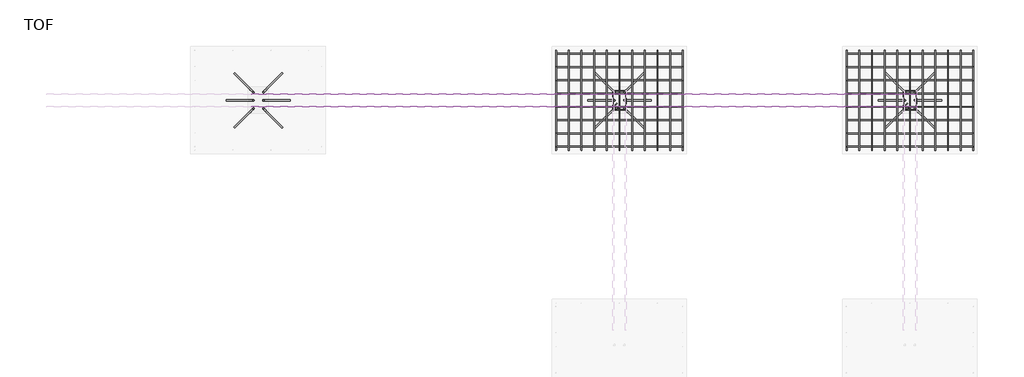
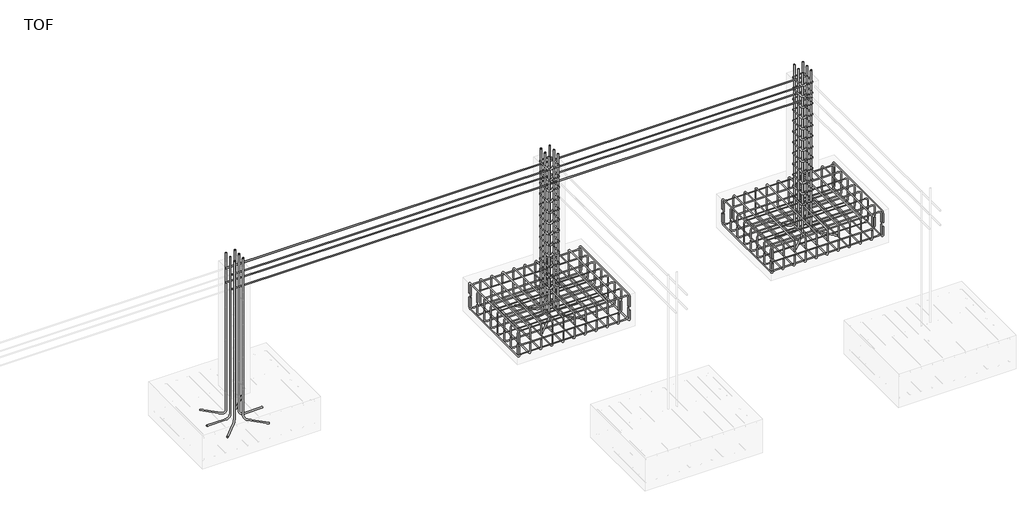
# One storey, part 10 of 10: 36 reinforcing bars.
"""IFC4 building model written with IfcOpenShell, lengths in millimetres."""

from ifc_helpers import new_model, si_unit, point, frame, origin, place, context, project, spatial, polyline, circle_curve, trimmed, segment, composite_curve, source, transform, mapped, element, save
from ifc_brep_helpers import swept_disk

model = new_model("IFC4")

# Units and contexts
model_context = context("Model", 3, world=origin())
ifc_project = project(units=[si_unit("LENGTHUNIT", "METRE", prefix="MILLI")], contexts=[model_context])

# Site, building, storey
site = spatial("IfcSite", under=ifc_project)
building = spatial("IfcBuilding", under=site)
storey = spatial("IfcBuildingStorey", under=building, Name="TOF", Elevation=-1828.8)

# Reinforcing bars
placement = place(None, origin())
reinforcing_bar_shape = source(origin(), model_context, "Body", "SolidModel", [
    swept_disk(composite_curve([segment(polyline([(10345.2782143, -7144.6267376, -2018.8), (10345.2782143, -7144.6267376, -1908.8)]), True, "CONTINUOUS"), segment(trimmed(circle_curve(frame((10345.2782143, -7179.6267376, -1908.8), z_axis=(1.0, 0.0, 0.0), x_axis=(0.0, 35.0, 0.0)), 35.0), [point((10345.2782143, -7144.6267376, -1908.8))], [point((10345.2782143, -7179.6267376, -1873.8))], True, "CARTESIAN"), True, "CONTINUOUS"), segment(polyline([(10345.2782143, -7179.6267376, -1873.8), (10345.2782143, -8219.6267376, -1873.8)]), True, "CONTINUOUS"), segment(trimmed(circle_curve(frame((10345.2782143, -8219.6267376, -1908.8), z_axis=(1.0, 0.0, 0.0), x_axis=(0.0, 0.0, 35.0)), 35.0), [point((10345.2782143, -8219.6267376, -1873.8))], [point((10345.2782143, -8254.6267376, -1908.8))], True, "CARTESIAN"), True, "CONTINUOUS"), segment(polyline([(10345.2782143, -8254.6267376, -1908.8), (10345.2782143, -8254.6267376, -2018.8)]), True, "CONTINUOUS")], self_intersect=False), 5.0),
])
element("IfcReinforcingBar", 1, at=placement, inside=storey, context=model_context, shape_type="MappedRepresentation", body=[
    mapped(reinforcing_bar_shape, transform((0.0, 0.0, 0.0), x_axis=(1.0, 0.0, 0.0), y_axis=(0.0, 1.0, 0.0), z_axis=(0.0, 0.0, 1.0))),
    mapped(reinforcing_bar_shape, transform((-141.0, 0.0, 0.0), x_axis=(1.0, 0.0, 0.0), y_axis=(0.0, 1.0, 0.0), z_axis=(0.0, 0.0, 1.0))),
    mapped(reinforcing_bar_shape, transform((-282.0, 0.0, 0.0), x_axis=(1.0, 0.0, 0.0), y_axis=(0.0, 1.0, 0.0), z_axis=(0.0, 0.0, 1.0))),
    mapped(reinforcing_bar_shape, transform((-423.0, 0.0, 0.0), x_axis=(1.0, 0.0, 0.0), y_axis=(0.0, 1.0, 0.0), z_axis=(0.0, 0.0, 1.0))),
    mapped(reinforcing_bar_shape, transform((-564.0, 0.0, 0.0), x_axis=(1.0, 0.0, 0.0), y_axis=(0.0, 1.0, 0.0), z_axis=(0.0, 0.0, 1.0))),
    mapped(reinforcing_bar_shape, transform((-705.0, 0.0, 0.0), x_axis=(1.0, 0.0, 0.0), y_axis=(0.0, 1.0, 0.0), z_axis=(0.0, 0.0, 1.0))),
    mapped(reinforcing_bar_shape, transform((-846.0, 0.0, 0.0), x_axis=(1.0, 0.0, 0.0), y_axis=(0.0, 1.0, 0.0), z_axis=(0.0, 0.0, 1.0))),
    mapped(reinforcing_bar_shape, transform((-987.0, 0.0, 0.0), x_axis=(1.0, 0.0, 0.0), y_axis=(0.0, 1.0, 0.0), z_axis=(0.0, 0.0, 1.0))),
    mapped(reinforcing_bar_shape, transform((-1128.0, 0.0, 0.0), x_axis=(1.0, 0.0, 0.0), y_axis=(0.0, 1.0, 0.0), z_axis=(0.0, 0.0, 1.0))),
    mapped(reinforcing_bar_shape, transform((-1269.0, 0.0, 0.0), x_axis=(1.0, 0.0, 0.0), y_axis=(0.0, 1.0, 0.0), z_axis=(0.0, 0.0, 1.0))),
    mapped(reinforcing_bar_shape, transform((-1410.0, 0.0, 0.0), x_axis=(1.0, 0.0, 0.0), y_axis=(0.0, 1.0, 0.0), z_axis=(0.0, 0.0, 1.0))),
])
reinforcing_bar_2_shape = source(origin(), model_context, "Body", "SolidModel", [
    swept_disk(composite_curve([segment(polyline([(10345.2782143, -8254.6267376, -2077.5233378), (10345.2782143, -8254.6267376, -2187.5233378)]), True, "CONTINUOUS"), segment(trimmed(circle_curve(frame((10345.2782143, -8219.6267376, -2187.5233378), z_axis=(1.0, 0.0, 0.0), x_axis=(0.0, -35.0, 0.0)), 35.0), [point((10345.2782143, -8254.6267376, -2187.5233378))], [point((10345.2782143, -8219.6267376, -2222.5233378))], True, "CARTESIAN"), True, "CONTINUOUS"), segment(polyline([(10345.2782143, -8219.6267376, -2222.5233378), (10345.2782143, -7179.6267376, -2222.5233378)]), True, "CONTINUOUS"), segment(trimmed(circle_curve(frame((10345.2782143, -7179.6267376, -2187.5233378), z_axis=(1.0, 0.0, 0.0), x_axis=(0.0, 0.0, -35.0)), 35.0), [point((10345.2782143, -7179.6267376, -2222.5233378))], [point((10345.2782143, -7144.6267376, -2187.5233378))], True, "CARTESIAN"), True, "CONTINUOUS"), segment(polyline([(10345.2782143, -7144.6267376, -2187.5233378), (10345.2782143, -7144.6267376, -2077.5233378)]), True, "CONTINUOUS")], self_intersect=False), 5.0),
])
element("IfcReinforcingBar", 2, at=placement, inside=storey, context=model_context, shape_type="MappedRepresentation", body=[
    mapped(reinforcing_bar_2_shape, transform((0.0, 0.0, 0.0), x_axis=(1.0, 0.0, 0.0), y_axis=(0.0, 1.0, 0.0), z_axis=(0.0, 0.0, 1.0))),
    mapped(reinforcing_bar_2_shape, transform((-141.0, 0.0, 0.0), x_axis=(1.0, 0.0, 0.0), y_axis=(0.0, 1.0, 0.0), z_axis=(0.0, 0.0, 1.0))),
    mapped(reinforcing_bar_2_shape, transform((-282.0, 0.0, 0.0), x_axis=(1.0, 0.0, 0.0), y_axis=(0.0, 1.0, 0.0), z_axis=(0.0, 0.0, 1.0))),
    mapped(reinforcing_bar_2_shape, transform((-423.0, 0.0, 0.0), x_axis=(1.0, 0.0, 0.0), y_axis=(0.0, 1.0, 0.0), z_axis=(0.0, 0.0, 1.0))),
    mapped(reinforcing_bar_2_shape, transform((-564.0, 0.0, 0.0), x_axis=(1.0, 0.0, 0.0), y_axis=(0.0, 1.0, 0.0), z_axis=(0.0, 0.0, 1.0))),
    mapped(reinforcing_bar_2_shape, transform((-705.0, 0.0, 0.0), x_axis=(1.0, 0.0, 0.0), y_axis=(0.0, 1.0, 0.0), z_axis=(0.0, 0.0, 1.0))),
    mapped(reinforcing_bar_2_shape, transform((-846.0, 0.0, 0.0), x_axis=(1.0, 0.0, 0.0), y_axis=(0.0, 1.0, 0.0), z_axis=(0.0, 0.0, 1.0))),
    mapped(reinforcing_bar_2_shape, transform((-987.0, 0.0, 0.0), x_axis=(1.0, 0.0, 0.0), y_axis=(0.0, 1.0, 0.0), z_axis=(0.0, 0.0, 1.0))),
    mapped(reinforcing_bar_2_shape, transform((-1128.0, 0.0, 0.0), x_axis=(1.0, 0.0, 0.0), y_axis=(0.0, 1.0, 0.0), z_axis=(0.0, 0.0, 1.0))),
    mapped(reinforcing_bar_2_shape, transform((-1269.0, 0.0, 0.0), x_axis=(1.0, 0.0, 0.0), y_axis=(0.0, 1.0, 0.0), z_axis=(0.0, 0.0, 1.0))),
    mapped(reinforcing_bar_2_shape, transform((-1410.0, 0.0, 0.0), x_axis=(1.0, 0.0, 0.0), y_axis=(0.0, 1.0, 0.0), z_axis=(0.0, 0.0, 1.0))),
])
reinforcing_bar_3_shape = source(origin(), model_context, "Body", "SolidModel", [
    swept_disk(composite_curve([segment(polyline([(10345.2782143, -7179.6861459, -2066.1776706), (10345.2782143, -7179.6861459, -2176.1776706)]), True, "CONTINUOUS"), segment(trimmed(circle_curve(frame((10310.2782143, -7179.6861459, -2176.1776706), z_axis=(0.0, 1.0, 0.0), x_axis=(35.0, 0.0, 0.0)), 35.0), [point((10345.2782143, -7179.6861459, -2176.1776706))], [point((10310.2782143, -7179.6861459, -2211.1776706))], True, "CARTESIAN"), True, "CONTINUOUS"), segment(polyline([(10310.2782143, -7179.6861459, -2211.1776706), (8970.2782143, -7179.6861459, -2211.1776706)]), True, "CONTINUOUS"), segment(trimmed(circle_curve(frame((8970.2782143, -7179.6861459, -2176.1776706), z_axis=(0.0, 1.0, 0.0), x_axis=(0.0, 0.0, -35.0)), 35.0), [point((8970.2782143, -7179.6861459, -2211.1776706))], [point((8935.2782143, -7179.6861459, -2176.1776706))], True, "CARTESIAN"), True, "CONTINUOUS"), segment(polyline([(8935.2782143, -7179.6861459, -2176.1776706), (8935.2782143, -7179.6861459, -2066.1776706)]), True, "CONTINUOUS")], self_intersect=False), 5.0),
])
element("IfcReinforcingBar", 3, at=placement, inside=storey, context=model_context, shape_type="MappedRepresentation", body=[
    mapped(reinforcing_bar_3_shape, transform((0.0, 0.0, 0.0), x_axis=(1.0, 0.0, 0.0), y_axis=(0.0, 1.0, 0.0), z_axis=(0.0, 0.0, 1.0))),
    mapped(reinforcing_bar_3_shape, transform((0.0, -148.0321606, 0.0), x_axis=(1.0, 0.0, 0.0), y_axis=(0.0, 1.0, 0.0), z_axis=(0.0, 0.0, 1.0))),
    mapped(reinforcing_bar_3_shape, transform((0.0, -296.0643211, 0.0), x_axis=(1.0, 0.0, 0.0), y_axis=(0.0, 1.0, 0.0), z_axis=(0.0, 0.0, 1.0))),
    mapped(reinforcing_bar_3_shape, transform((0.0, -444.0964817, 0.0), x_axis=(1.0, 0.0, 0.0), y_axis=(0.0, 1.0, 0.0), z_axis=(0.0, 0.0, 1.0))),
    mapped(reinforcing_bar_3_shape, transform((0.0, -592.1286423, 0.0), x_axis=(1.0, 0.0, 0.0), y_axis=(0.0, 1.0, 0.0), z_axis=(0.0, 0.0, 1.0))),
    mapped(reinforcing_bar_3_shape, transform((0.0, -740.1608029, 0.0), x_axis=(1.0, 0.0, 0.0), y_axis=(0.0, 1.0, 0.0), z_axis=(0.0, 0.0, 1.0))),
    mapped(reinforcing_bar_3_shape, transform((0.0, -888.1929634, 0.0), x_axis=(1.0, 0.0, 0.0), y_axis=(0.0, 1.0, 0.0), z_axis=(0.0, 0.0, 1.0))),
    mapped(reinforcing_bar_3_shape, transform((0.0, -1036.225124, 0.0), x_axis=(1.0, 0.0, 0.0), y_axis=(0.0, 1.0, 0.0), z_axis=(0.0, 0.0, 1.0))),
])
reinforcing_bar_4_shape = source(origin(), model_context, "Body", "SolidModel", [
    swept_disk(composite_curve([segment(polyline([(10345.2782143, -8215.9112699, -2039.256778), (10345.2782143, -8215.9112699, -1929.256778)]), True, "CONTINUOUS"), segment(trimmed(circle_curve(frame((10310.2782143, -8215.9112699, -1929.256778), z_axis=(0.0, -1.0, 0.0), x_axis=(35.0, 0.0, 0.0)), 35.0), [point((10345.2782143, -8215.9112699, -1929.256778))], [point((10310.2782143, -8215.9112699, -1894.256778))], True, "CARTESIAN"), True, "CONTINUOUS"), segment(polyline([(10310.2782143, -8215.9112699, -1894.256778), (8970.2782143, -8215.9112699, -1894.256778)]), True, "CONTINUOUS"), segment(trimmed(circle_curve(frame((8970.2782143, -8215.9112699, -1929.256778), z_axis=(0.0, -1.0, 0.0), x_axis=(0.0, 0.0, 35.0)), 35.0), [point((8970.2782143, -8215.9112699, -1894.256778))], [point((8935.2782143, -8215.9112699, -1929.256778))], True, "CARTESIAN"), True, "CONTINUOUS"), segment(polyline([(8935.2782143, -8215.9112699, -1929.256778), (8935.2782143, -8215.9112699, -2039.256778)]), True, "CONTINUOUS")], self_intersect=False), 5.0),
])
element("IfcReinforcingBar", 4, at=placement, inside=storey, context=model_context, shape_type="MappedRepresentation", body=[
    mapped(reinforcing_bar_4_shape, transform((0.0, 0.0, 0.0), x_axis=(1.0, 0.0, 0.0), y_axis=(0.0, 1.0, 0.0), z_axis=(0.0, 0.0, 1.0))),
    mapped(reinforcing_bar_4_shape, transform((0.0, 148.0321606, 0.0), x_axis=(1.0, 0.0, 0.0), y_axis=(0.0, 1.0, 0.0), z_axis=(0.0, 0.0, 1.0))),
    mapped(reinforcing_bar_4_shape, transform((0.0, 296.0643211, 0.0), x_axis=(1.0, 0.0, 0.0), y_axis=(0.0, 1.0, 0.0), z_axis=(0.0, 0.0, 1.0))),
    mapped(reinforcing_bar_4_shape, transform((0.0, 444.0964817, 0.0), x_axis=(1.0, 0.0, 0.0), y_axis=(0.0, 1.0, 0.0), z_axis=(0.0, 0.0, 1.0))),
    mapped(reinforcing_bar_4_shape, transform((0.0, 592.1286423, 0.0), x_axis=(1.0, 0.0, 0.0), y_axis=(0.0, 1.0, 0.0), z_axis=(0.0, 0.0, 1.0))),
    mapped(reinforcing_bar_4_shape, transform((0.0, 740.1608029, 0.0), x_axis=(1.0, 0.0, 0.0), y_axis=(0.0, 1.0, 0.0), z_axis=(0.0, 0.0, 1.0))),
    mapped(reinforcing_bar_4_shape, transform((0.0, 888.1929634, 0.0), x_axis=(1.0, 0.0, 0.0), y_axis=(0.0, 1.0, 0.0), z_axis=(0.0, 0.0, 1.0))),
    mapped(reinforcing_bar_4_shape, transform((0.0, 1036.225124, 0.0), x_axis=(1.0, 0.0, 0.0), y_axis=(0.0, 1.0, 0.0), z_axis=(0.0, 0.0, 1.0))),
])
reinforcing_bar_5_shape = source(origin(), model_context, "Body", "SolidModel", [
    swept_disk(composite_curve([segment(polyline([(13575.2782143, -7144.6267376, -2018.8), (13575.2782143, -7144.6267376, -1908.8)]), True, "CONTINUOUS"), segment(trimmed(circle_curve(frame((13575.2782143, -7179.6267376, -1908.8), z_axis=(1.0, 0.0, 0.0), x_axis=(0.0, 35.0, 0.0)), 35.0), [point((13575.2782143, -7144.6267376, -1908.8))], [point((13575.2782143, -7179.6267376, -1873.8))], True, "CARTESIAN"), True, "CONTINUOUS"), segment(polyline([(13575.2782143, -7179.6267376, -1873.8), (13575.2782143, -8219.6267376, -1873.8)]), True, "CONTINUOUS"), segment(trimmed(circle_curve(frame((13575.2782143, -8219.6267376, -1908.8), z_axis=(1.0, 0.0, 0.0), x_axis=(0.0, 0.0, 35.0)), 35.0), [point((13575.2782143, -8219.6267376, -1873.8))], [point((13575.2782143, -8254.6267376, -1908.8))], True, "CARTESIAN"), True, "CONTINUOUS"), segment(polyline([(13575.2782143, -8254.6267376, -1908.8), (13575.2782143, -8254.6267376, -2018.8)]), True, "CONTINUOUS")], self_intersect=False), 5.0),
])
element("IfcReinforcingBar", 5, at=placement, inside=storey, context=model_context, shape_type="MappedRepresentation", body=[
    mapped(reinforcing_bar_5_shape, transform((0.0, 0.0, 0.0), x_axis=(1.0, 0.0, 0.0), y_axis=(0.0, 1.0, 0.0), z_axis=(0.0, 0.0, 1.0))),
    mapped(reinforcing_bar_5_shape, transform((-141.0, 0.0, 0.0), x_axis=(1.0, 0.0, 0.0), y_axis=(0.0, 1.0, 0.0), z_axis=(0.0, 0.0, 1.0))),
    mapped(reinforcing_bar_5_shape, transform((-282.0, 0.0, 0.0), x_axis=(1.0, 0.0, 0.0), y_axis=(0.0, 1.0, 0.0), z_axis=(0.0, 0.0, 1.0))),
    mapped(reinforcing_bar_5_shape, transform((-423.0, 0.0, 0.0), x_axis=(1.0, 0.0, 0.0), y_axis=(0.0, 1.0, 0.0), z_axis=(0.0, 0.0, 1.0))),
    mapped(reinforcing_bar_5_shape, transform((-564.0, 0.0, 0.0), x_axis=(1.0, 0.0, 0.0), y_axis=(0.0, 1.0, 0.0), z_axis=(0.0, 0.0, 1.0))),
    mapped(reinforcing_bar_5_shape, transform((-705.0, 0.0, 0.0), x_axis=(1.0, 0.0, 0.0), y_axis=(0.0, 1.0, 0.0), z_axis=(0.0, 0.0, 1.0))),
    mapped(reinforcing_bar_5_shape, transform((-846.0, 0.0, 0.0), x_axis=(1.0, 0.0, 0.0), y_axis=(0.0, 1.0, 0.0), z_axis=(0.0, 0.0, 1.0))),
    mapped(reinforcing_bar_5_shape, transform((-987.0, 0.0, 0.0), x_axis=(1.0, 0.0, 0.0), y_axis=(0.0, 1.0, 0.0), z_axis=(0.0, 0.0, 1.0))),
    mapped(reinforcing_bar_5_shape, transform((-1128.0, 0.0, 0.0), x_axis=(1.0, 0.0, 0.0), y_axis=(0.0, 1.0, 0.0), z_axis=(0.0, 0.0, 1.0))),
    mapped(reinforcing_bar_5_shape, transform((-1269.0, 0.0, 0.0), x_axis=(1.0, 0.0, 0.0), y_axis=(0.0, 1.0, 0.0), z_axis=(0.0, 0.0, 1.0))),
    mapped(reinforcing_bar_5_shape, transform((-1410.0, 0.0, 0.0), x_axis=(1.0, 0.0, 0.0), y_axis=(0.0, 1.0, 0.0), z_axis=(0.0, 0.0, 1.0))),
])
reinforcing_bar_6_shape = source(origin(), model_context, "Body", "SolidModel", [
    swept_disk(composite_curve([segment(polyline([(13575.2782143, -8254.6267376, -2077.5233378), (13575.2782143, -8254.6267376, -2187.5233378)]), True, "CONTINUOUS"), segment(trimmed(circle_curve(frame((13575.2782143, -8219.6267376, -2187.5233378), z_axis=(1.0, 0.0, 0.0), x_axis=(0.0, -35.0, 0.0)), 35.0), [point((13575.2782143, -8254.6267376, -2187.5233378))], [point((13575.2782143, -8219.6267376, -2222.5233378))], True, "CARTESIAN"), True, "CONTINUOUS"), segment(polyline([(13575.2782143, -8219.6267376, -2222.5233378), (13575.2782143, -7179.6267376, -2222.5233378)]), True, "CONTINUOUS"), segment(trimmed(circle_curve(frame((13575.2782143, -7179.6267376, -2187.5233378), z_axis=(1.0, 0.0, 0.0), x_axis=(0.0, 0.0, -35.0)), 35.0), [point((13575.2782143, -7179.6267376, -2222.5233378))], [point((13575.2782143, -7144.6267376, -2187.5233378))], True, "CARTESIAN"), True, "CONTINUOUS"), segment(polyline([(13575.2782143, -7144.6267376, -2187.5233378), (13575.2782143, -7144.6267376, -2077.5233378)]), True, "CONTINUOUS")], self_intersect=False), 5.0),
])
element("IfcReinforcingBar", 6, at=placement, inside=storey, context=model_context, shape_type="MappedRepresentation", body=[
    mapped(reinforcing_bar_6_shape, transform((0.0, 0.0, 0.0), x_axis=(1.0, 0.0, 0.0), y_axis=(0.0, 1.0, 0.0), z_axis=(0.0, 0.0, 1.0))),
    mapped(reinforcing_bar_6_shape, transform((-141.0, 0.0, 0.0), x_axis=(1.0, 0.0, 0.0), y_axis=(0.0, 1.0, 0.0), z_axis=(0.0, 0.0, 1.0))),
    mapped(reinforcing_bar_6_shape, transform((-282.0, 0.0, 0.0), x_axis=(1.0, 0.0, 0.0), y_axis=(0.0, 1.0, 0.0), z_axis=(0.0, 0.0, 1.0))),
    mapped(reinforcing_bar_6_shape, transform((-423.0, 0.0, 0.0), x_axis=(1.0, 0.0, 0.0), y_axis=(0.0, 1.0, 0.0), z_axis=(0.0, 0.0, 1.0))),
    mapped(reinforcing_bar_6_shape, transform((-564.0, 0.0, 0.0), x_axis=(1.0, 0.0, 0.0), y_axis=(0.0, 1.0, 0.0), z_axis=(0.0, 0.0, 1.0))),
    mapped(reinforcing_bar_6_shape, transform((-705.0, 0.0, 0.0), x_axis=(1.0, 0.0, 0.0), y_axis=(0.0, 1.0, 0.0), z_axis=(0.0, 0.0, 1.0))),
    mapped(reinforcing_bar_6_shape, transform((-846.0, 0.0, 0.0), x_axis=(1.0, 0.0, 0.0), y_axis=(0.0, 1.0, 0.0), z_axis=(0.0, 0.0, 1.0))),
    mapped(reinforcing_bar_6_shape, transform((-987.0, 0.0, 0.0), x_axis=(1.0, 0.0, 0.0), y_axis=(0.0, 1.0, 0.0), z_axis=(0.0, 0.0, 1.0))),
    mapped(reinforcing_bar_6_shape, transform((-1128.0, 0.0, 0.0), x_axis=(1.0, 0.0, 0.0), y_axis=(0.0, 1.0, 0.0), z_axis=(0.0, 0.0, 1.0))),
    mapped(reinforcing_bar_6_shape, transform((-1269.0, 0.0, 0.0), x_axis=(1.0, 0.0, 0.0), y_axis=(0.0, 1.0, 0.0), z_axis=(0.0, 0.0, 1.0))),
    mapped(reinforcing_bar_6_shape, transform((-1410.0, 0.0, 0.0), x_axis=(1.0, 0.0, 0.0), y_axis=(0.0, 1.0, 0.0), z_axis=(0.0, 0.0, 1.0))),
])
reinforcing_bar_7_shape = source(origin(), model_context, "Body", "SolidModel", [
    swept_disk(composite_curve([segment(polyline([(13575.2782143, -7179.6861459, -2066.1776706), (13575.2782143, -7179.6861459, -2176.1776706)]), True, "CONTINUOUS"), segment(trimmed(circle_curve(frame((13540.2782143, -7179.6861459, -2176.1776706), z_axis=(0.0, 1.0, 0.0), x_axis=(35.0, 0.0, 0.0)), 35.0), [point((13575.2782143, -7179.6861459, -2176.1776706))], [point((13540.2782143, -7179.6861459, -2211.1776706))], True, "CARTESIAN"), True, "CONTINUOUS"), segment(polyline([(13540.2782143, -7179.6861459, -2211.1776706), (12200.2782143, -7179.6861459, -2211.1776706)]), True, "CONTINUOUS"), segment(trimmed(circle_curve(frame((12200.2782143, -7179.6861459, -2176.1776706), z_axis=(0.0, 1.0, 0.0), x_axis=(0.0, 0.0, -35.0)), 35.0), [point((12200.2782143, -7179.6861459, -2211.1776706))], [point((12165.2782143, -7179.6861459, -2176.1776706))], True, "CARTESIAN"), True, "CONTINUOUS"), segment(polyline([(12165.2782143, -7179.6861459, -2176.1776706), (12165.2782143, -7179.6861459, -2066.1776706)]), True, "CONTINUOUS")], self_intersect=False), 5.0),
])
element("IfcReinforcingBar", 7, at=placement, inside=storey, context=model_context, shape_type="MappedRepresentation", body=[
    mapped(reinforcing_bar_7_shape, transform((0.0, 0.0, 0.0), x_axis=(1.0, 0.0, 0.0), y_axis=(0.0, 1.0, 0.0), z_axis=(0.0, 0.0, 1.0))),
    mapped(reinforcing_bar_7_shape, transform((0.0, -148.0321606, 0.0), x_axis=(1.0, 0.0, 0.0), y_axis=(0.0, 1.0, 0.0), z_axis=(0.0, 0.0, 1.0))),
    mapped(reinforcing_bar_7_shape, transform((0.0, -296.0643211, 0.0), x_axis=(1.0, 0.0, 0.0), y_axis=(0.0, 1.0, 0.0), z_axis=(0.0, 0.0, 1.0))),
    mapped(reinforcing_bar_7_shape, transform((0.0, -444.0964817, 0.0), x_axis=(1.0, 0.0, 0.0), y_axis=(0.0, 1.0, 0.0), z_axis=(0.0, 0.0, 1.0))),
    mapped(reinforcing_bar_7_shape, transform((0.0, -592.1286423, 0.0), x_axis=(1.0, 0.0, 0.0), y_axis=(0.0, 1.0, 0.0), z_axis=(0.0, 0.0, 1.0))),
    mapped(reinforcing_bar_7_shape, transform((0.0, -740.1608029, 0.0), x_axis=(1.0, 0.0, 0.0), y_axis=(0.0, 1.0, 0.0), z_axis=(0.0, 0.0, 1.0))),
    mapped(reinforcing_bar_7_shape, transform((0.0, -888.1929634, 0.0), x_axis=(1.0, 0.0, 0.0), y_axis=(0.0, 1.0, 0.0), z_axis=(0.0, 0.0, 1.0))),
    mapped(reinforcing_bar_7_shape, transform((0.0, -1036.225124, 0.0), x_axis=(1.0, 0.0, 0.0), y_axis=(0.0, 1.0, 0.0), z_axis=(0.0, 0.0, 1.0))),
])
reinforcing_bar_8_shape = source(origin(), model_context, "Body", "SolidModel", [
    swept_disk(composite_curve([segment(polyline([(13575.2782143, -8215.9112699, -2039.256778), (13575.2782143, -8215.9112699, -1929.256778)]), True, "CONTINUOUS"), segment(trimmed(circle_curve(frame((13540.2782143, -8215.9112699, -1929.256778), z_axis=(0.0, -1.0, 0.0), x_axis=(35.0, 0.0, 0.0)), 35.0), [point((13575.2782143, -8215.9112699, -1929.256778))], [point((13540.2782143, -8215.9112699, -1894.256778))], True, "CARTESIAN"), True, "CONTINUOUS"), segment(polyline([(13540.2782143, -8215.9112699, -1894.256778), (12200.2782143, -8215.9112699, -1894.256778)]), True, "CONTINUOUS"), segment(trimmed(circle_curve(frame((12200.2782143, -8215.9112699, -1929.256778), z_axis=(0.0, -1.0, 0.0), x_axis=(0.0, 0.0, 35.0)), 35.0), [point((12200.2782143, -8215.9112699, -1894.256778))], [point((12165.2782143, -8215.9112699, -1929.256778))], True, "CARTESIAN"), True, "CONTINUOUS"), segment(polyline([(12165.2782143, -8215.9112699, -1929.256778), (12165.2782143, -8215.9112699, -2039.256778)]), True, "CONTINUOUS")], self_intersect=False), 5.0),
])
element("IfcReinforcingBar", 8, at=placement, inside=storey, context=model_context, shape_type="MappedRepresentation", body=[
    mapped(reinforcing_bar_8_shape, transform((0.0, 0.0, 0.0), x_axis=(1.0, 0.0, 0.0), y_axis=(0.0, 1.0, 0.0), z_axis=(0.0, 0.0, 1.0))),
    mapped(reinforcing_bar_8_shape, transform((0.0, 148.0321606, 0.0), x_axis=(1.0, 0.0, 0.0), y_axis=(0.0, 1.0, 0.0), z_axis=(0.0, 0.0, 1.0))),
    mapped(reinforcing_bar_8_shape, transform((0.0, 296.0643211, 0.0), x_axis=(1.0, 0.0, 0.0), y_axis=(0.0, 1.0, 0.0), z_axis=(0.0, 0.0, 1.0))),
    mapped(reinforcing_bar_8_shape, transform((0.0, 444.0964817, 0.0), x_axis=(1.0, 0.0, 0.0), y_axis=(0.0, 1.0, 0.0), z_axis=(0.0, 0.0, 1.0))),
    mapped(reinforcing_bar_8_shape, transform((0.0, 592.1286423, 0.0), x_axis=(1.0, 0.0, 0.0), y_axis=(0.0, 1.0, 0.0), z_axis=(0.0, 0.0, 1.0))),
    mapped(reinforcing_bar_8_shape, transform((0.0, 740.1608029, 0.0), x_axis=(1.0, 0.0, 0.0), y_axis=(0.0, 1.0, 0.0), z_axis=(0.0, 0.0, 1.0))),
    mapped(reinforcing_bar_8_shape, transform((0.0, 888.1929634, 0.0), x_axis=(1.0, 0.0, 0.0), y_axis=(0.0, 1.0, 0.0), z_axis=(0.0, 0.0, 1.0))),
    mapped(reinforcing_bar_8_shape, transform((0.0, 1036.225124, 0.0), x_axis=(1.0, 0.0, 0.0), y_axis=(0.0, 1.0, 0.0), z_axis=(0.0, 0.0, 1.0))),
])
element("IfcReinforcingBar", 9, at=placement, inside=storey, context=model_context, shape_type="SolidModel", body=[
    swept_disk(composite_curve([segment(polyline([(5680.884816, -7790.2333393, -20.0), (5680.884816, -7790.2333393, -2138.7824747)]), True, "CONTINUOUS"), segment(trimmed(circle_curve(frame((5720.1292424, -7829.4777657, -2138.7824747), z_axis=(-0.7071067811865545, -0.7071067811865406, 0.0), x_axis=(-39.24442640000052, 39.24442640000052, 0.0)), 55.5), [point((5680.884816, -7790.2333393, -2138.7824747))], [point((5720.1292424, -7829.4777657, -2194.2824747))], True, "CARTESIAN"), True, "CONTINUOUS"), segment(polyline([(5720.1292424, -7829.4777657, -2194.2824747), (5892.5083915, -8001.8569148, -2194.2824747)]), True, "CONTINUOUS")], self_intersect=False), 8.0),
])
element("IfcReinforcingBar", 10, at=placement, inside=storey, context=model_context, shape_type="SolidModel", body=[
    swept_disk(composite_curve([segment(polyline([(5680.934816, -7699.6267376, -20.0), (5680.934816, -7699.6267376, -2138.7824747)]), True, "CONTINUOUS"), segment(trimmed(circle_curve(frame((5736.434816, -7699.6267376, -2138.7824747), z_axis=(0.0, -1.0, 0.0), x_axis=(-55.5, 0.0, 0.0)), 55.5), [point((5680.934816, -7699.6267376, -2138.7824747))], [point((5736.434816, -7699.6267376, -2194.2824747))], True, "CARTESIAN"), True, "CONTINUOUS"), segment(polyline([(5736.434816, -7699.6267376, -2194.2824747), (5980.1657466, -7699.6267376, -2194.2824747)]), True, "CONTINUOUS")], self_intersect=False), 8.0),
])
element("IfcReinforcingBar", 11, at=placement, inside=storey, context=model_context, shape_type="SolidModel", body=[
    swept_disk(composite_curve([segment(polyline([(5680.884816, -7609.0201359, -20.0), (5680.884816, -7609.0201359, -2138.7824747)]), True, "CONTINUOUS"), segment(trimmed(circle_curve(frame((5720.1292424, -7569.7757095, -2138.7824747), z_axis=(0.7071067811865545, -0.7071067811865407, 0.0), x_axis=(-39.24442640000052, -39.24442640000052, 0.0)), 55.5), [point((5680.884816, -7609.0201359, -2138.7824747))], [point((5720.1292424, -7569.7757095, -2194.2824747))], True, "CARTESIAN"), True, "CONTINUOUS"), segment(polyline([(5720.1292424, -7569.7757095, -2194.2824747), (5892.5083915, -7397.3965603, -2194.2824747)]), True, "CONTINUOUS")], self_intersect=False), 8.0),
])
element("IfcReinforcingBar", 12, at=placement, inside=storey, context=model_context, shape_type="SolidModel", body=[
    swept_disk(composite_curve([segment(polyline([(5569.6716126, -7790.2333393, -20.0), (5569.6716126, -7790.2333393, -2138.7824747)]), True, "CONTINUOUS"), segment(trimmed(circle_curve(frame((5530.4271862, -7829.4777657, -2138.7824747), z_axis=(-0.7071067811865517, 0.7071067811865434, 0.0), x_axis=(39.24442640000052, 39.24442640000052, 0.0)), 55.5), [point((5569.6716126, -7790.2333393, -2138.7824747))], [point((5530.4271862, -7829.4777657, -2194.2824747))], True, "CARTESIAN"), True, "CONTINUOUS"), segment(polyline([(5530.4271862, -7829.4777657, -2194.2824747), (5358.048037, -8001.8569148, -2194.2824747)]), True, "CONTINUOUS")], self_intersect=False), 8.0),
])
element("IfcReinforcingBar", 13, at=placement, inside=storey, context=model_context, shape_type="SolidModel", body=[
    swept_disk(composite_curve([segment(polyline([(5569.6216126, -7699.6267376, -20.0), (5569.6216126, -7699.6267376, -2138.7824747)]), True, "CONTINUOUS"), segment(trimmed(circle_curve(frame((5514.1216126, -7699.6267376, -2138.7824747), z_axis=(0.0, 1.0, 0.0), x_axis=(55.5, 0.0, 0.0)), 55.5), [point((5569.6216126, -7699.6267376, -2138.7824747))], [point((5514.1216126, -7699.6267376, -2194.2824747))], True, "CARTESIAN"), True, "CONTINUOUS"), segment(polyline([(5514.1216126, -7699.6267376, -2194.2824747), (5270.3906819, -7699.6267376, -2194.2824747)]), True, "CONTINUOUS")], self_intersect=False), 8.0),
])
element("IfcReinforcingBar", 14, at=placement, inside=storey, context=model_context, shape_type="SolidModel", body=[
    swept_disk(composite_curve([segment(polyline([(5569.6716126, -7609.0201359, -20.0), (5569.6716126, -7609.0201359, -2138.7824747)]), True, "CONTINUOUS"), segment(trimmed(circle_curve(frame((5530.4271862, -7569.7757095, -2138.7824747), z_axis=(0.7071067811865572, 0.7071067811865379, 0.0), x_axis=(39.24442640000052, -39.24442640000052, 0.0)), 55.5), [point((5569.6716126, -7609.0201359, -2138.7824747))], [point((5530.4271862, -7569.7757095, -2194.2824747))], True, "CARTESIAN"), True, "CONTINUOUS"), segment(polyline([(5530.4271862, -7569.7757095, -2194.2824747), (5358.048037, -7397.3965603, -2194.2824747)]), True, "CONTINUOUS")], self_intersect=False), 8.0),
])
reinforcing_bar_9_shape = source(origin(), model_context, "Body", "SolidModel", [
    swept_disk(composite_curve([segment(polyline([(9610.248777, -7730.7150493, -1784.8), (9576.3076515, -7764.6561748, -1784.8)]), True, "CONTINUOUS"), segment(trimmed(circle_curve(frame((9593.2782143, -7781.6267376, -1784.8), z_axis=(0.0, 0.0, 1.0), x_axis=(-16.970562800001062, 16.970562799999243, 0.0)), 24.0), [point((9576.3076515, -7764.6561748, -1784.8))], [point((9593.2782143, -7805.6267376, -1784.8))], True, "CARTESIAN"), True, "CONTINUOUS"), segment(polyline([(9593.2782143, -7805.6267376, -1784.8), (9687.2782143, -7805.6267376, -1784.8)]), True, "CONTINUOUS"), segment(trimmed(circle_curve(frame((9687.2782143, -7781.6267376, -1784.8), z_axis=(0.0, 0.0, 1.0), x_axis=(0.0, -24.0, 0.0)), 24.0), [point((9687.2782143, -7805.6267376, -1784.8))], [point((9711.2782143, -7781.6267376, -1784.8))], True, "CARTESIAN"), True, "CONTINUOUS"), segment(polyline([(9711.2782143, -7781.6267376, -1784.8), (9711.2782143, -7617.6267376, -1784.8)]), True, "CONTINUOUS"), segment(trimmed(circle_curve(frame((9687.3162115, -7617.6267376, -1786.149972), z_axis=(-0.05624883273897078, 0.0, 0.9984167811167355), x_axis=(23.962002800000846, 0.0, 1.3499719999999797)), 24.0), [point((9711.2782143, -7617.6267376, -1784.8))], [point((9687.3162115, -7593.6267376, -1786.149972))], True, "CARTESIAN"), True, "CONTINUOUS"), segment(polyline([(9687.3162115, -7593.6267376, -1786.149972), (9593.240217, -7593.6267376, -1791.450028)]), True, "CONTINUOUS"), segment(trimmed(circle_curve(frame((9593.240217, -7617.6267376, -1791.450028), z_axis=(-0.05624883273897078, 0.0, 0.9984167811167355), x_axis=(0.0, 24.0, 0.0)), 24.0), [point((9593.240217, -7593.6267376, -1791.450028))], [point((9569.2782143, -7617.6267376, -1792.8))], True, "CARTESIAN"), True, "CONTINUOUS"), segment(polyline([(9569.2782143, -7617.6267376, -1792.8), (9569.2782143, -7781.6267376, -1792.8)]), True, "CONTINUOUS"), segment(trimmed(circle_curve(frame((9593.2782143, -7781.6267376, -1792.8), z_axis=(0.0, 0.0, 1.0), x_axis=(-24.0, 0.0, 0.0)), 24.0), [point((9569.2782143, -7781.6267376, -1792.8))], [point((9610.248777, -7798.5973003, -1792.8))], True, "CARTESIAN"), True, "CONTINUOUS"), segment(polyline([(9610.248777, -7798.5973003, -1792.8), (9644.1899025, -7764.6561748, -1792.8)]), True, "CONTINUOUS")], self_intersect=False), 4.0),
])
element("IfcReinforcingBar", 15, at=placement, inside=storey, context=model_context, shape_type="MappedRepresentation", body=[
    mapped(reinforcing_bar_9_shape, transform((0.0, 0.0, 0.0), x_axis=(1.0, 0.0, 0.0), y_axis=(0.0, 1.0, 0.0), z_axis=(0.0, 0.0, 1.0))),
    mapped(reinforcing_bar_9_shape, transform((0.0, 0.0, 145.9395608), x_axis=(1.0, 0.0, 0.0), y_axis=(0.0, 1.0, 0.0), z_axis=(0.0, 0.0, 1.0))),
    mapped(reinforcing_bar_9_shape, transform((0.0, 0.0, 291.8791216), x_axis=(1.0, 0.0, 0.0), y_axis=(0.0, 1.0, 0.0), z_axis=(0.0, 0.0, 1.0))),
    mapped(reinforcing_bar_9_shape, transform((0.0, 0.0, 437.8186825), x_axis=(1.0, 0.0, 0.0), y_axis=(0.0, 1.0, 0.0), z_axis=(0.0, 0.0, 1.0))),
    mapped(reinforcing_bar_9_shape, transform((0.0, 0.0, 583.7582433), x_axis=(1.0, 0.0, 0.0), y_axis=(0.0, 1.0, 0.0), z_axis=(0.0, 0.0, 1.0))),
    mapped(reinforcing_bar_9_shape, transform((0.0, 0.0, 729.6978041), x_axis=(1.0, 0.0, 0.0), y_axis=(0.0, 1.0, 0.0), z_axis=(0.0, 0.0, 1.0))),
    mapped(reinforcing_bar_9_shape, transform((0.0, 0.0, 875.6373649), x_axis=(1.0, 0.0, 0.0), y_axis=(0.0, 1.0, 0.0), z_axis=(0.0, 0.0, 1.0))),
    mapped(reinforcing_bar_9_shape, transform((0.0, 0.0, 1021.5769258), x_axis=(1.0, 0.0, 0.0), y_axis=(0.0, 1.0, 0.0), z_axis=(0.0, 0.0, 1.0))),
    mapped(reinforcing_bar_9_shape, transform((0.0, 0.0, 1167.5164866), x_axis=(1.0, 0.0, 0.0), y_axis=(0.0, 1.0, 0.0), z_axis=(0.0, 0.0, 1.0))),
    mapped(reinforcing_bar_9_shape, transform((0.0, 0.0, 1313.4560474), x_axis=(1.0, 0.0, 0.0), y_axis=(0.0, 1.0, 0.0), z_axis=(0.0, 0.0, 1.0))),
    mapped(reinforcing_bar_9_shape, transform((0.0, 0.0, 1459.3956082), x_axis=(1.0, 0.0, 0.0), y_axis=(0.0, 1.0, 0.0), z_axis=(0.0, 0.0, 1.0))),
    mapped(reinforcing_bar_9_shape, transform((0.0, 0.0, 1605.3351691), x_axis=(1.0, 0.0, 0.0), y_axis=(0.0, 1.0, 0.0), z_axis=(0.0, 0.0, 1.0))),
])
element("IfcReinforcingBar", 16, at=placement, inside=storey, context=model_context, shape_type="SolidModel", body=[
    swept_disk(composite_curve([segment(polyline([(9695.884816, -7790.2333393, -20.0), (9695.884816, -7790.2333393, -2138.7824747)]), True, "CONTINUOUS"), segment(trimmed(circle_curve(frame((9735.1292424, -7829.4777657, -2138.7824747), z_axis=(-0.7071067811865545, -0.7071067811865406, 0.0), x_axis=(-39.24442640000052, 39.24442640000052, 0.0)), 55.5), [point((9695.884816, -7790.2333393, -2138.7824747))], [point((9735.1292424, -7829.4777657, -2194.2824747))], True, "CARTESIAN"), True, "CONTINUOUS"), segment(polyline([(9735.1292424, -7829.4777657, -2194.2824747), (9907.5083915, -8001.8569148, -2194.2824747)]), True, "CONTINUOUS")], self_intersect=False), 8.0),
])
element("IfcReinforcingBar", 17, at=placement, inside=storey, context=model_context, shape_type="SolidModel", body=[
    swept_disk(composite_curve([segment(polyline([(9695.934816, -7699.6267376, -20.0), (9695.934816, -7699.6267376, -2138.7824747)]), True, "CONTINUOUS"), segment(trimmed(circle_curve(frame((9751.434816, -7699.6267376, -2138.7824747), z_axis=(0.0, -1.0, 0.0), x_axis=(-55.5, 0.0, 0.0)), 55.5), [point((9695.934816, -7699.6267376, -2138.7824747))], [point((9751.434816, -7699.6267376, -2194.2824747))], True, "CARTESIAN"), True, "CONTINUOUS"), segment(polyline([(9751.434816, -7699.6267376, -2194.2824747), (9995.1657466, -7699.6267376, -2194.2824747)]), True, "CONTINUOUS")], self_intersect=False), 8.0),
])
element("IfcReinforcingBar", 18, at=placement, inside=storey, context=model_context, shape_type="SolidModel", body=[
    swept_disk(composite_curve([segment(polyline([(9695.884816, -7609.0201359, -20.0), (9695.884816, -7609.0201359, -2138.7824747)]), True, "CONTINUOUS"), segment(trimmed(circle_curve(frame((9735.1292424, -7569.7757095, -2138.7824747), z_axis=(0.7071067811865545, -0.7071067811865407, 0.0), x_axis=(-39.24442640000052, -39.24442640000052, 0.0)), 55.5), [point((9695.884816, -7609.0201359, -2138.7824747))], [point((9735.1292424, -7569.7757095, -2194.2824747))], True, "CARTESIAN"), True, "CONTINUOUS"), segment(polyline([(9735.1292424, -7569.7757095, -2194.2824747), (9907.5083915, -7397.3965603, -2194.2824747)]), True, "CONTINUOUS")], self_intersect=False), 8.0),
])
element("IfcReinforcingBar", 19, at=placement, inside=storey, context=model_context, shape_type="SolidModel", body=[
    swept_disk(composite_curve([segment(polyline([(9584.6716126, -7790.2333393, -20.0), (9584.6716126, -7790.2333393, -2138.7824747)]), True, "CONTINUOUS"), segment(trimmed(circle_curve(frame((9545.4271862, -7829.4777657, -2138.7824747), z_axis=(-0.7071067811865517, 0.7071067811865434, 0.0), x_axis=(39.2444263999987, 39.24442640000052, 0.0)), 55.5), [point((9584.6716126, -7790.2333393, -2138.7824747))], [point((9545.4271862, -7829.4777657, -2194.2824747))], True, "CARTESIAN"), True, "CONTINUOUS"), segment(polyline([(9545.4271862, -7829.4777657, -2194.2824747), (9373.048037, -8001.8569148, -2194.2824747)]), True, "CONTINUOUS")], self_intersect=False), 8.0),
])
element("IfcReinforcingBar", 20, at=placement, inside=storey, context=model_context, shape_type="SolidModel", body=[
    swept_disk(composite_curve([segment(polyline([(9584.6216126, -7699.6267376, -20.0), (9584.6216126, -7699.6267376, -2138.7824747)]), True, "CONTINUOUS"), segment(trimmed(circle_curve(frame((9529.1216126, -7699.6267376, -2138.7824747), z_axis=(0.0, 1.0, 0.0), x_axis=(55.5, 0.0, 0.0)), 55.5), [point((9584.6216126, -7699.6267376, -2138.7824747))], [point((9529.1216126, -7699.6267376, -2194.2824747))], True, "CARTESIAN"), True, "CONTINUOUS"), segment(polyline([(9529.1216126, -7699.6267376, -2194.2824747), (9285.3906819, -7699.6267376, -2194.2824747)]), True, "CONTINUOUS")], self_intersect=False), 8.0),
])
element("IfcReinforcingBar", 21, at=placement, inside=storey, context=model_context, shape_type="SolidModel", body=[
    swept_disk(composite_curve([segment(polyline([(9584.6716126, -7609.0201359, -20.0), (9584.6716126, -7609.0201359, -2138.7824747)]), True, "CONTINUOUS"), segment(trimmed(circle_curve(frame((9545.4271862, -7569.7757095, -2138.7824747), z_axis=(0.7071067811865572, 0.7071067811865379, 0.0), x_axis=(39.2444263999987, -39.24442640000052, 0.0)), 55.5), [point((9584.6716126, -7609.0201359, -2138.7824747))], [point((9545.4271862, -7569.7757095, -2194.2824747))], True, "CARTESIAN"), True, "CONTINUOUS"), segment(polyline([(9545.4271862, -7569.7757095, -2194.2824747), (9373.048037, -7397.3965603, -2194.2824747)]), True, "CONTINUOUS")], self_intersect=False), 8.0),
])
reinforcing_bar_10_shape = source(origin(), model_context, "Body", "SolidModel", [
    swept_disk(composite_curve([segment(polyline([(12840.248777, -7730.7150493, -1784.8), (12806.3076515, -7764.6561748, -1784.8)]), True, "CONTINUOUS"), segment(trimmed(circle_curve(frame((12823.2782143, -7781.6267376, -1784.8), z_axis=(0.0, 0.0, 1.0), x_axis=(-16.970562800001062, 16.970562799999243, 0.0)), 24.0), [point((12806.3076515, -7764.6561748, -1784.8))], [point((12823.2782143, -7805.6267376, -1784.8))], True, "CARTESIAN"), True, "CONTINUOUS"), segment(polyline([(12823.2782143, -7805.6267376, -1784.8), (12917.2782143, -7805.6267376, -1784.8)]), True, "CONTINUOUS"), segment(trimmed(circle_curve(frame((12917.2782143, -7781.6267376, -1784.8), z_axis=(0.0, 0.0, 1.0), x_axis=(0.0, -24.0, 0.0)), 24.0), [point((12917.2782143, -7805.6267376, -1784.8))], [point((12941.2782143, -7781.6267376, -1784.8))], True, "CARTESIAN"), True, "CONTINUOUS"), segment(polyline([(12941.2782143, -7781.6267376, -1784.8), (12941.2782143, -7617.6267376, -1784.8)]), True, "CONTINUOUS"), segment(trimmed(circle_curve(frame((12917.3162115, -7617.6267376, -1786.149972), z_axis=(-0.05624883273897078, 0.0, 0.9984167811167355), x_axis=(23.962002800000846, 0.0, 1.3499719999999797)), 24.0), [point((12941.2782143, -7617.6267376, -1784.8))], [point((12917.3162115, -7593.6267376, -1786.149972))], True, "CARTESIAN"), True, "CONTINUOUS"), segment(polyline([(12917.3162115, -7593.6267376, -1786.149972), (12823.240217, -7593.6267376, -1791.450028)]), True, "CONTINUOUS"), segment(trimmed(circle_curve(frame((12823.240217, -7617.6267376, -1791.450028), z_axis=(-0.05624883273897078, 0.0, 0.9984167811167355), x_axis=(0.0, 24.0, 0.0)), 24.0), [point((12823.240217, -7593.6267376, -1791.450028))], [point((12799.2782143, -7617.6267376, -1792.8))], True, "CARTESIAN"), True, "CONTINUOUS"), segment(polyline([(12799.2782143, -7617.6267376, -1792.8), (12799.2782143, -7781.6267376, -1792.8)]), True, "CONTINUOUS"), segment(trimmed(circle_curve(frame((12823.2782143, -7781.6267376, -1792.8), z_axis=(0.0, 0.0, 1.0), x_axis=(-24.0, 0.0, 0.0)), 24.0), [point((12799.2782143, -7781.6267376, -1792.8))], [point((12840.248777, -7798.5973003, -1792.8))], True, "CARTESIAN"), True, "CONTINUOUS"), segment(polyline([(12840.248777, -7798.5973003, -1792.8), (12874.1899025, -7764.6561748, -1792.8)]), True, "CONTINUOUS")], self_intersect=False), 4.0),
])
element("IfcReinforcingBar", 22, at=placement, inside=storey, context=model_context, shape_type="MappedRepresentation", body=[
    mapped(reinforcing_bar_10_shape, transform((0.0, 0.0, 0.0), x_axis=(1.0, 0.0, 0.0), y_axis=(0.0, 1.0, 0.0), z_axis=(0.0, 0.0, 1.0))),
    mapped(reinforcing_bar_10_shape, transform((0.0, 0.0, 145.9395608), x_axis=(1.0, 0.0, 0.0), y_axis=(0.0, 1.0, 0.0), z_axis=(0.0, 0.0, 1.0))),
    mapped(reinforcing_bar_10_shape, transform((0.0, 0.0, 291.8791216), x_axis=(1.0, 0.0, 0.0), y_axis=(0.0, 1.0, 0.0), z_axis=(0.0, 0.0, 1.0))),
    mapped(reinforcing_bar_10_shape, transform((0.0, 0.0, 437.8186825), x_axis=(1.0, 0.0, 0.0), y_axis=(0.0, 1.0, 0.0), z_axis=(0.0, 0.0, 1.0))),
    mapped(reinforcing_bar_10_shape, transform((0.0, 0.0, 583.7582433), x_axis=(1.0, 0.0, 0.0), y_axis=(0.0, 1.0, 0.0), z_axis=(0.0, 0.0, 1.0))),
    mapped(reinforcing_bar_10_shape, transform((0.0, 0.0, 729.6978041), x_axis=(1.0, 0.0, 0.0), y_axis=(0.0, 1.0, 0.0), z_axis=(0.0, 0.0, 1.0))),
    mapped(reinforcing_bar_10_shape, transform((0.0, 0.0, 875.6373649), x_axis=(1.0, 0.0, 0.0), y_axis=(0.0, 1.0, 0.0), z_axis=(0.0, 0.0, 1.0))),
    mapped(reinforcing_bar_10_shape, transform((0.0, 0.0, 1021.5769258), x_axis=(1.0, 0.0, 0.0), y_axis=(0.0, 1.0, 0.0), z_axis=(0.0, 0.0, 1.0))),
    mapped(reinforcing_bar_10_shape, transform((0.0, 0.0, 1167.5164866), x_axis=(1.0, 0.0, 0.0), y_axis=(0.0, 1.0, 0.0), z_axis=(0.0, 0.0, 1.0))),
    mapped(reinforcing_bar_10_shape, transform((0.0, 0.0, 1313.4560474), x_axis=(1.0, 0.0, 0.0), y_axis=(0.0, 1.0, 0.0), z_axis=(0.0, 0.0, 1.0))),
    mapped(reinforcing_bar_10_shape, transform((0.0, 0.0, 1459.3956082), x_axis=(1.0, 0.0, 0.0), y_axis=(0.0, 1.0, 0.0), z_axis=(0.0, 0.0, 1.0))),
    mapped(reinforcing_bar_10_shape, transform((0.0, 0.0, 1605.3351691), x_axis=(1.0, 0.0, 0.0), y_axis=(0.0, 1.0, 0.0), z_axis=(0.0, 0.0, 1.0))),
])
element("IfcReinforcingBar", 23, at=placement, inside=storey, context=model_context, shape_type="SolidModel", body=[
    swept_disk(composite_curve([segment(polyline([(12925.884816, -7790.2333393, -20.0), (12925.884816, -7790.2333393, -2138.7824747)]), True, "CONTINUOUS"), segment(trimmed(circle_curve(frame((12965.1292424, -7829.4777657, -2138.7824747), z_axis=(-0.7071067811865545, -0.7071067811865406, 0.0), x_axis=(-39.24442640000052, 39.24442640000052, 0.0)), 55.5), [point((12925.884816, -7790.2333393, -2138.7824747))], [point((12965.1292424, -7829.4777657, -2194.2824747))], True, "CARTESIAN"), True, "CONTINUOUS"), segment(polyline([(12965.1292424, -7829.4777657, -2194.2824747), (13137.5083915, -8001.8569148, -2194.2824747)]), True, "CONTINUOUS")], self_intersect=False), 8.0),
])
element("IfcReinforcingBar", 24, at=placement, inside=storey, context=model_context, shape_type="SolidModel", body=[
    swept_disk(composite_curve([segment(polyline([(12925.934816, -7699.6267376, -20.0), (12925.934816, -7699.6267376, -2138.7824747)]), True, "CONTINUOUS"), segment(trimmed(circle_curve(frame((12981.434816, -7699.6267376, -2138.7824747), z_axis=(0.0, -1.0, 0.0), x_axis=(-55.5, 0.0, 0.0)), 55.5), [point((12925.934816, -7699.6267376, -2138.7824747))], [point((12981.434816, -7699.6267376, -2194.2824747))], True, "CARTESIAN"), True, "CONTINUOUS"), segment(polyline([(12981.434816, -7699.6267376, -2194.2824747), (13225.1657466, -7699.6267376, -2194.2824747)]), True, "CONTINUOUS")], self_intersect=False), 8.0),
])
element("IfcReinforcingBar", 25, at=placement, inside=storey, context=model_context, shape_type="SolidModel", body=[
    swept_disk(composite_curve([segment(polyline([(12925.884816, -7609.0201359, -20.0), (12925.884816, -7609.0201359, -2138.7824747)]), True, "CONTINUOUS"), segment(trimmed(circle_curve(frame((12965.1292424, -7569.7757095, -2138.7824747), z_axis=(0.7071067811865545, -0.7071067811865407, 0.0), x_axis=(-39.24442640000052, -39.24442640000052, 0.0)), 55.5), [point((12925.884816, -7609.0201359, -2138.7824747))], [point((12965.1292424, -7569.7757095, -2194.2824747))], True, "CARTESIAN"), True, "CONTINUOUS"), segment(polyline([(12965.1292424, -7569.7757095, -2194.2824747), (13137.5083915, -7397.3965603, -2194.2824747)]), True, "CONTINUOUS")], self_intersect=False), 8.0),
])
element("IfcReinforcingBar", 26, at=placement, inside=storey, context=model_context, shape_type="SolidModel", body=[
    swept_disk(composite_curve([segment(polyline([(12814.6716126, -7790.2333393, -20.0), (12814.6716126, -7790.2333393, -2138.7824747)]), True, "CONTINUOUS"), segment(trimmed(circle_curve(frame((12775.4271862, -7829.4777657, -2138.7824747), z_axis=(-0.7071067811865517, 0.7071067811865434, 0.0), x_axis=(39.2444263999987, 39.24442640000052, 0.0)), 55.5), [point((12814.6716126, -7790.2333393, -2138.7824747))], [point((12775.4271862, -7829.4777657, -2194.2824747))], True, "CARTESIAN"), True, "CONTINUOUS"), segment(polyline([(12775.4271862, -7829.4777657, -2194.2824747), (12603.048037, -8001.8569148, -2194.2824747)]), True, "CONTINUOUS")], self_intersect=False), 8.0),
])
element("IfcReinforcingBar", 27, at=placement, inside=storey, context=model_context, shape_type="SolidModel", body=[
    swept_disk(composite_curve([segment(polyline([(12814.6216126, -7699.6267376, -20.0), (12814.6216126, -7699.6267376, -2138.7824747)]), True, "CONTINUOUS"), segment(trimmed(circle_curve(frame((12759.1216126, -7699.6267376, -2138.7824747), z_axis=(0.0, 1.0, 0.0), x_axis=(55.5, 0.0, 0.0)), 55.5), [point((12814.6216126, -7699.6267376, -2138.7824747))], [point((12759.1216126, -7699.6267376, -2194.2824747))], True, "CARTESIAN"), True, "CONTINUOUS"), segment(polyline([(12759.1216126, -7699.6267376, -2194.2824747), (12515.3906819, -7699.6267376, -2194.2824747)]), True, "CONTINUOUS")], self_intersect=False), 8.0),
])
element("IfcReinforcingBar", 28, at=placement, inside=storey, context=model_context, shape_type="SolidModel", body=[
    swept_disk(composite_curve([segment(polyline([(12814.6716126, -7609.0201359, -20.0), (12814.6716126, -7609.0201359, -2138.7824747)]), True, "CONTINUOUS"), segment(trimmed(circle_curve(frame((12775.4271862, -7569.7757095, -2138.7824747), z_axis=(0.7071067811865572, 0.7071067811865379, 0.0), x_axis=(39.2444263999987, -39.24442640000052, 0.0)), 55.5), [point((12814.6716126, -7609.0201359, -2138.7824747))], [point((12775.4271862, -7569.7757095, -2194.2824747))], True, "CARTESIAN"), True, "CONTINUOUS"), segment(polyline([(12775.4271862, -7569.7757095, -2194.2824747), (12603.048037, -7397.3965603, -2194.2824747)]), True, "CONTINUOUS")], self_intersect=False), 8.0),
])
element("IfcReinforcingBar", 29, at=placement, inside=storey, context=model_context, shape_type="SolidModel", body=[
    swept_disk(composite_curve([segment(polyline([(9715.2782143, -7769.5917105, -210.0508449), (5550.2782143, -7769.5917105, -210.0508449)]), True, "CONTINUOUS")], self_intersect=False), 6.0),
])
element("IfcReinforcingBar", 30, at=placement, inside=storey, context=model_context, shape_type="SolidModel", body=[
    swept_disk(composite_curve([segment(polyline([(9715.2782143, -7769.5917105, -405.0508449), (5550.2782143, -7769.5917105, -405.0508449)]), True, "CONTINUOUS")], self_intersect=False), 6.0),
])
element("IfcReinforcingBar", 31, at=placement, inside=storey, context=model_context, shape_type="SolidModel", body=[
    swept_disk(composite_curve([segment(polyline([(9715.2782143, -7629.6617646, -210.0508449), (5550.2782143, -7629.6617646, -210.0508449)]), True, "CONTINUOUS")], self_intersect=False), 6.0),
])
element("IfcReinforcingBar", 32, at=placement, inside=storey, context=model_context, shape_type="SolidModel", body=[
    swept_disk(composite_curve([segment(polyline([(9715.2782143, -7629.6617646, -405.0508449), (5550.2782143, -7629.6617646, -405.0508449)]), True, "CONTINUOUS")], self_intersect=False), 6.0),
])
element("IfcReinforcingBar", 33, at=placement, inside=storey, context=model_context, shape_type="SolidModel", body=[
    swept_disk(composite_curve([segment(polyline([(12945.2782143, -7769.5917105, -210.0508449), (9565.2782143, -7769.5917105, -210.0508449)]), True, "CONTINUOUS")], self_intersect=False), 6.0),
])
element("IfcReinforcingBar", 34, at=placement, inside=storey, context=model_context, shape_type="SolidModel", body=[
    swept_disk(composite_curve([segment(polyline([(12945.2782143, -7769.5917105, -405.0508449), (9565.2782143, -7769.5917105, -405.0508449)]), True, "CONTINUOUS")], self_intersect=False), 6.0),
])
element("IfcReinforcingBar", 35, at=placement, inside=storey, context=model_context, shape_type="SolidModel", body=[
    swept_disk(composite_curve([segment(polyline([(12945.2782143, -7629.6617646, -210.0508449), (9565.2782143, -7629.6617646, -210.0508449)]), True, "CONTINUOUS")], self_intersect=False), 6.0),
])
element("IfcReinforcingBar", 36, at=placement, inside=storey, context=model_context, shape_type="SolidModel", body=[
    swept_disk(composite_curve([segment(polyline([(12945.2782143, -7629.6617646, -405.0508449), (9565.2782143, -7629.6617646, -405.0508449)]), True, "CONTINUOUS")], self_intersect=False), 6.0),
])

save(model, "model.ifc")

# Revit data of these elements
# Elements 1, 2, 3, 4, 5, 6, 7, 8, 9, 10, 11, 12, 13, 14, 15, 16, 17, 18, 19, 20, 21, 22, 23, 24, 25, 26, 27, 28, 29, 30, 31, 32, 33, 34, 35, 36 (IfcReinforcingBar)
#   Phase Created = New Construction
